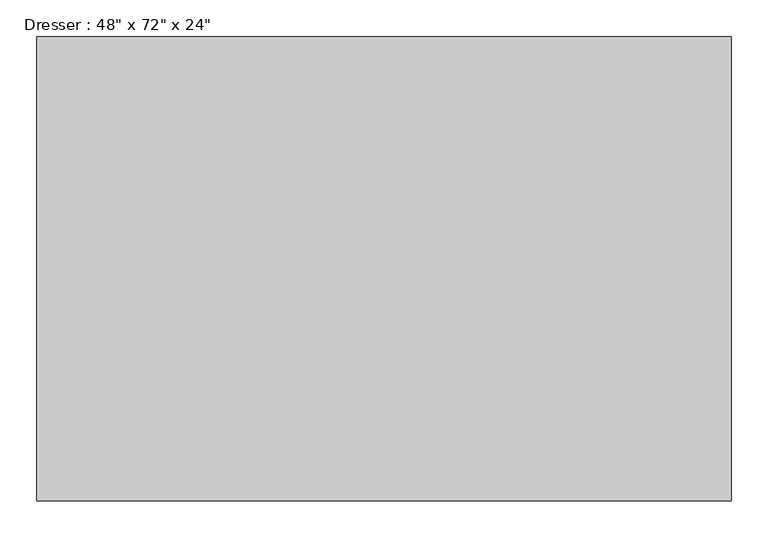
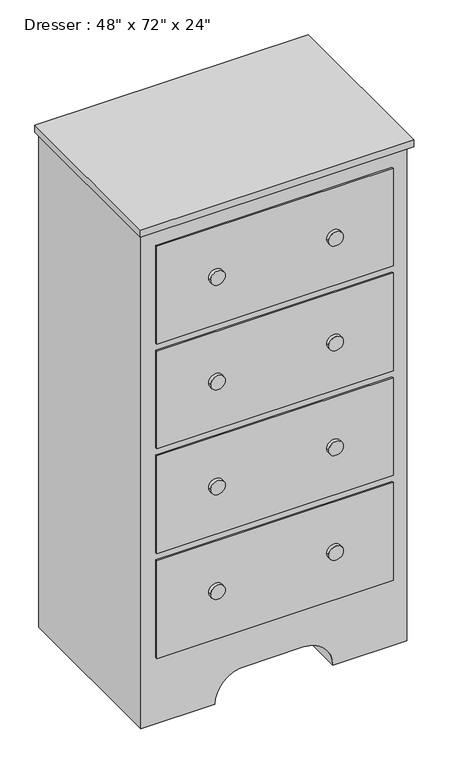
"""IFC4 building model written with IfcOpenShell, lengths in millimetres: furniture geometry."""

from ifc_helpers import new_model, si_unit, point, frame, frame_2d, origin, place, context, project, spatial, polyline, circle_curve, trimmed, segment, composite_curve, outline, extrude, source, transform, mapped, element, save


def furniture_33655958(model_context):
    return source(origin(), model_context, "Body", "SweptSolid", [
        extrude(outline(polyline([(200.7067402, -58.3629541), (200.7067402, -687.0129541), (-739.0932598, -687.0129541), (-739.0932598, -58.3629541), (200.7067402, -58.3629541)])), frame((0.0, 0.0, 1803.4), z_axis=(0.0, 0.0, 1.0), x_axis=(1.0, 0.0, 0.0)), (0.0, 0.0, 1.0), 25.4),
        extrude(outline(composite_curve([segment(polyline([(0.0, 188.0067402), (1803.4, 188.0067402), (1803.4, -726.3932598), (0.0, -726.3932598), (0.0, -472.3932598)]), True, "CONTINUOUS"), segment(trimmed(circle_curve(frame_2d((0.0, -370.7932598)), 101.6), [point((0.0, -472.3932598))], [point((101.6, -370.7932598))], True, "CARTESIAN"), True, "CONTINUOUS"), segment(polyline([(101.6, -370.7932598), (101.6, -167.5932598)]), True, "CONTINUOUS"), segment(trimmed(circle_curve(frame_2d((0.0, -167.5932598)), 101.6), [point((101.6, -167.5932598))], [point((0.0, -65.9932598))], True, "CARTESIAN"), True, "CONTINUOUS"), segment(polyline([(0.0, -65.9932598), (0.0, 188.0067402)]), True, "CONTINUOUS")], self_intersect=False)), frame((0.0, -667.9629541, 0.0), z_axis=(0.0, 1.0, 0.0), x_axis=(0.0, 0.0, 1.0)), (0.0, 0.0, 1.0), 609.6),
        extrude(outline(composite_curve([segment(trimmed(circle_curve(frame_2d((1562.1, -65.9932598)), 25.4), [point((1562.1, -91.3932598))], [point((1562.1, -40.5932598))], False, "CARTESIAN"), True, "CONTINUOUS"), segment(trimmed(circle_curve(frame_2d((1562.1, -65.9932598)), 25.4), [point((1562.1, -40.5932598))], [point((1562.1, -91.3932598))], False, "CARTESIAN"), True, "CONTINUOUS")], self_intersect=False)), frame((0.0, -687.0129541, 0.0), z_axis=(0.0, 1.0, 0.0), x_axis=(0.0, 0.0, 1.0)), (0.0, 0.0, 1.0), 12.7),
        extrude(outline(composite_curve([segment(trimmed(circle_curve(frame_2d((1181.1, -65.9932598)), 25.4), [point((1181.1, -91.3932598))], [point((1181.1, -40.5932598))], False, "CARTESIAN"), True, "CONTINUOUS"), segment(trimmed(circle_curve(frame_2d((1181.1, -65.9932598)), 25.4), [point((1181.1, -40.5932598))], [point((1181.1, -91.3932598))], False, "CARTESIAN"), True, "CONTINUOUS")], self_intersect=False)), frame((0.0, -687.0129541, 0.0), z_axis=(0.0, 1.0, 0.0), x_axis=(0.0, 0.0, 1.0)), (0.0, 0.0, 1.0), 12.7),
        extrude(outline(composite_curve([segment(trimmed(circle_curve(frame_2d((800.1, -65.9932598)), 25.4), [point((800.1, -91.3932598))], [point((800.1, -40.5932598))], False, "CARTESIAN"), True, "CONTINUOUS"), segment(trimmed(circle_curve(frame_2d((800.1, -65.9932598)), 25.4), [point((800.1, -40.5932598))], [point((800.1, -91.3932598))], False, "CARTESIAN"), True, "CONTINUOUS")], self_intersect=False)), frame((0.0, -687.0129541, 0.0), z_axis=(0.0, 1.0, 0.0), x_axis=(0.0, 0.0, 1.0)), (0.0, 0.0, 1.0), 12.7),
        extrude(outline(composite_curve([segment(trimmed(circle_curve(frame_2d((419.1, -65.9932598)), 25.4), [point((419.1, -91.3932598))], [point((419.1, -40.5932598))], False, "CARTESIAN"), True, "CONTINUOUS"), segment(trimmed(circle_curve(frame_2d((419.1, -65.9932598)), 25.4), [point((419.1, -40.5932598))], [point((419.1, -91.3932598))], False, "CARTESIAN"), True, "CONTINUOUS")], self_intersect=False)), frame((0.0, -687.0129541, 0.0), z_axis=(0.0, 1.0, 0.0), x_axis=(0.0, 0.0, 1.0)), (0.0, 0.0, 1.0), 12.7),
        extrude(outline(composite_curve([segment(trimmed(circle_curve(frame_2d((419.1, -472.3932598)), 25.4), [point((419.1, -497.7932598))], [point((419.1, -446.9932598))], False, "CARTESIAN"), True, "CONTINUOUS"), segment(trimmed(circle_curve(frame_2d((419.1, -472.3932598)), 25.4), [point((419.1, -446.9932598))], [point((419.1, -497.7932598))], False, "CARTESIAN"), True, "CONTINUOUS")], self_intersect=False)), frame((0.0, -687.0129541, 0.0), z_axis=(0.0, 1.0, 0.0), x_axis=(0.0, 0.0, 1.0)), (0.0, 0.0, 1.0), 12.7),
        extrude(outline(composite_curve([segment(trimmed(circle_curve(frame_2d((800.1, -472.3932598)), 25.4), [point((800.1, -497.7932598))], [point((800.1, -446.9932598))], False, "CARTESIAN"), True, "CONTINUOUS"), segment(trimmed(circle_curve(frame_2d((800.1, -472.3932598)), 25.4), [point((800.1, -446.9932598))], [point((800.1, -497.7932598))], False, "CARTESIAN"), True, "CONTINUOUS")], self_intersect=False)), frame((0.0, -687.0129541, 0.0), z_axis=(0.0, 1.0, 0.0), x_axis=(0.0, 0.0, 1.0)), (0.0, 0.0, 1.0), 12.7),
        extrude(outline(composite_curve([segment(trimmed(circle_curve(frame_2d((1181.1, -472.3932598)), 25.4), [point((1181.1, -497.7932598))], [point((1181.1, -446.9932598))], False, "CARTESIAN"), True, "CONTINUOUS"), segment(trimmed(circle_curve(frame_2d((1181.1, -472.3932598)), 25.4), [point((1181.1, -446.9932598))], [point((1181.1, -497.7932598))], False, "CARTESIAN"), True, "CONTINUOUS")], self_intersect=False)), frame((0.0, -687.0129541, 0.0), z_axis=(0.0, 1.0, 0.0), x_axis=(0.0, 0.0, 1.0)), (0.0, 0.0, 1.0), 12.7),
        extrude(outline(composite_curve([segment(trimmed(circle_curve(frame_2d((1562.1, -472.3932598)), 25.4), [point((1562.1, -497.7932598))], [point((1562.1, -446.9932598))], False, "CARTESIAN"), True, "CONTINUOUS"), segment(trimmed(circle_curve(frame_2d((1562.1, -472.3932598)), 25.4), [point((1562.1, -446.9932598))], [point((1562.1, -497.7932598))], False, "CARTESIAN"), True, "CONTINUOUS")], self_intersect=False)), frame((0.0, -687.0129541, 0.0), z_axis=(0.0, 1.0, 0.0), x_axis=(0.0, 0.0, 1.0)), (0.0, 0.0, 1.0), 12.7),
        extrude(outline(polyline([(137.2067402, -674.3129541), (-675.5932598, -674.3129541), (-675.5932598, -667.9629541), (137.2067402, -667.9629541), (137.2067402, -674.3129541)])), frame((0.0, 0.0, 1384.3), z_axis=(0.0, 0.0, 1.0), x_axis=(1.0, 0.0, 0.0)), (0.0, 0.0, 1.0), 355.6),
        extrude(outline(polyline([(137.2067402, -674.3129541), (-675.5932598, -674.3129541), (-675.5932598, -667.9629541), (137.2067402, -667.9629541), (137.2067402, -674.3129541)])), frame((0.0, 0.0, 1003.3), z_axis=(0.0, 0.0, 1.0), x_axis=(1.0, 0.0, 0.0)), (0.0, 0.0, 1.0), 355.6),
        extrude(outline(polyline([(137.2067402, -674.3129541), (-675.5932598, -674.3129541), (-675.5932598, -667.9629541), (137.2067402, -667.9629541), (137.2067402, -674.3129541)])), frame((0.0, 0.0, 622.3), z_axis=(0.0, 0.0, 1.0), x_axis=(1.0, 0.0, 0.0)), (0.0, 0.0, 1.0), 355.6),
        extrude(outline(polyline([(137.2067402, -674.3129541), (-675.5932598, -674.3129541), (-675.5932598, -667.9629541), (137.2067402, -667.9629541), (137.2067402, -674.3129541)])), frame((0.0, 0.0, 241.3), z_axis=(0.0, 0.0, 1.0), x_axis=(1.0, 0.0, 0.0)), (0.0, 0.0, 1.0), 355.6),
    ])


if __name__ == "__main__":
    model = new_model("IFC4")
    model_context = context("Model", 3, world=origin())
    ifc_project = project(units=[si_unit("LENGTHUNIT", "METRE", prefix="MILLI")], contexts=[model_context])
    site = spatial("IfcSite", under=ifc_project)
    building = spatial("IfcBuilding", under=site)
    placement = place(None, origin())
    furniture_shape = furniture_33655958(model_context)
    element("IfcFurniture", 1, ObjectType="Dresser : 48\" x 72\" x 24\"", at=placement, inside=building, context=model_context, shape_type="MappedRepresentation", body=[
        mapped(furniture_shape, transform((0.0, 0.0, 0.0), x_axis=(1.0, 0.0, 0.0), y_axis=(0.0, 1.0, 0.0), z_axis=(0.0, 0.0, 1.0))),
    ])
    save(model, "model.ifc")

# Revit data of these elements
# Type "Dresser : 48\" x 72\" x 24\""
#   Assembly Code = "E2020200"
#   Depth = 2' - 0"
#   Height = 6' - 0"
#   Width = 3' - 0"
#   Dresser Material = Laminate - Ivory, Glossy
#   Drawer Material = Laminate, Ivory, Matte
#   Knob Material = Cherry
#   Default Elevation = 0
# Element 1 (IfcFurniture, "Dresser : 48\" x 72\" x 24\"")
#   Materials on its faces: "Laminate, Ivory, Matte", "Cherry", "Laminate - Ivory, Glossy"
# Materials
#   "Laminate - Ivory, Glossy": colour RGB 247 247 239, transparency 0
#   "Laminate, Ivory, Matte": class "Plastic", colour RGB 247 247 239, transparency 0, Description = "Plastic Laminate - Ivory, Matte", Cost = 0
#   "Cherry": class "Wood", colour RGB 226 177 128, transparency 0, Description = "Prunus Serotina", Cost = 0
